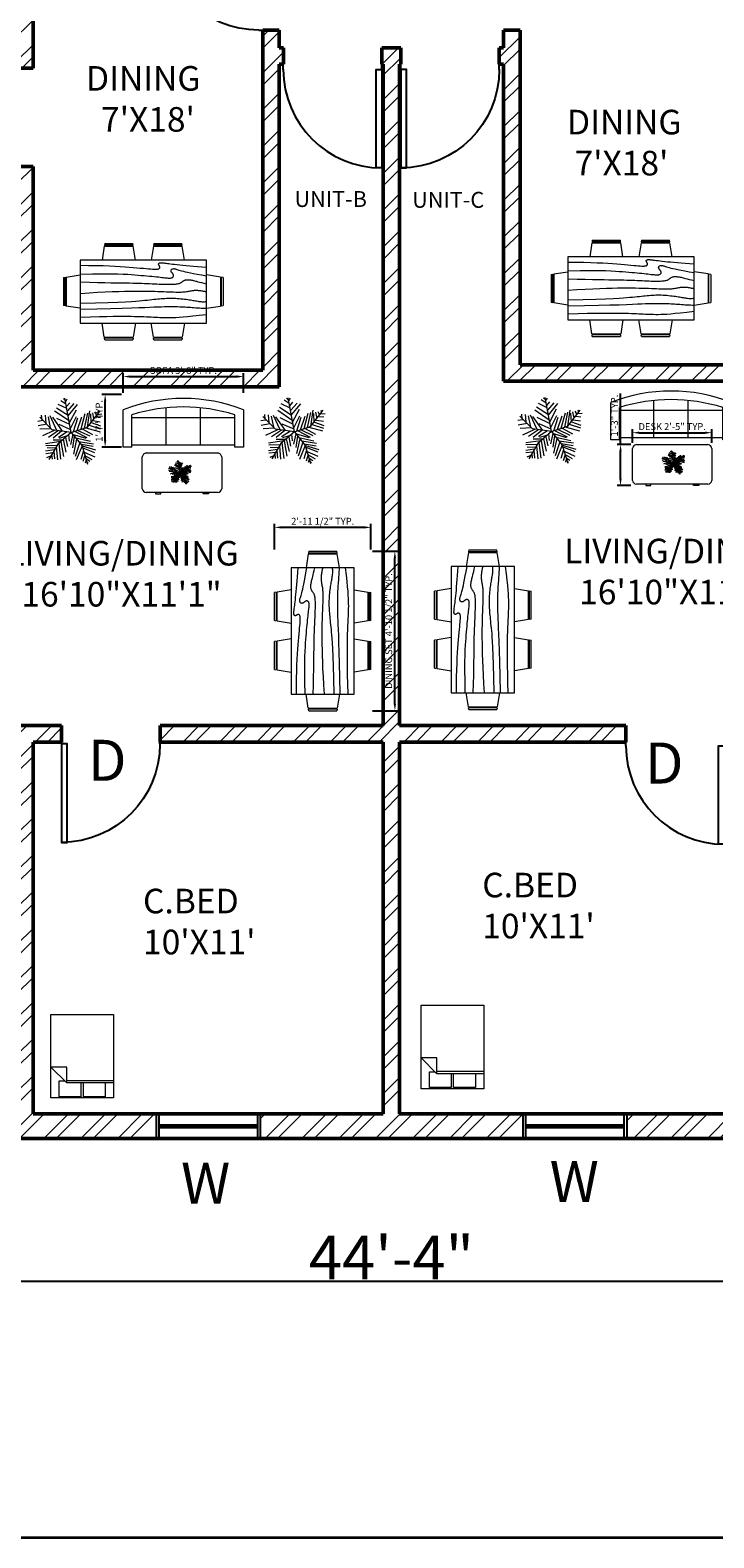
# Model space of a CAD drawing. Units: inches. Extents: x -31842 to -29388, y 18869 to 19743.
# Tile 2 of 12: x -31517 to -31268, y 18869 to 19420. Entities that reach past the tile are written whole.
import ezdxf

# ---------------------------------------------------------------- set-up
doc = ezdxf.new("R2010")
doc.units = ezdxf.units.IN
for name, color, linetype, lineweight in [('A-ANNO-DIMS', 2, 'Continuous', 18), ('A-ANNO-SYMB', 2, 'Continuous', 18), ('A-ANNO-TTLB', 7, 'Continuous', 35), ('A-AREA-IDEN', 3, 'Continuous', 18), ('A-DOOR', 3, 'Continuous', 25), ('A-FURN', 8, 'Continuous', 18), ('A-GLAZ', 4, 'Continuous', 25), ('A-WALL', 7, 'Continuous', 50), ('A-WALL-PATT', 8, 'Continuous', 13), ('L-PLNT', 3, 'Continuous', 13)]:
    doc.layers.add(name, color=color, linetype=linetype, lineweight=lineweight)
doc.styles.get("Standard").update_dxf_attribs({"font": 'arial.ttf'})
doc.dimstyles.new('ISO-25', dxfattribs={"dimtxt": 2.5, "dimasz": 2.5, "dimexe": 1.25, "dimexo": 0.625, "dimtad": 1, "dimdec": 0, "dimlunit": 3, "dimtxsty": 'Standard', "dimcen": 2.5, "dimadec": 0, "dimazin": 0, "dimtfac": 1, "dimtdec": 0, "dimtmove": 0, "dimatfit": 3, "dimfxl": 1, "dimarcsym": 0})

# ---------------------------------------------------------------- blocks, each defined once
blk = doc.blocks.new('*U8')
for p, q in [((0, 0), (0, -100)), ((750, 0), (750, -100))]:
    blk.add_line(p, q)
blk.add_lwpolyline([(0, 0), (0, 750), (43.75, 750), (43.75, 0)], close=True)
blk.add_arc((0, 0), 750, 0, 90)
blk = doc.blocks.new('Bed - Queen')
for p, q in [((0, -80.00003), (0, 0)), ((0, 0), (59.99999, 0)), ((59.99999, 0), (59.99999, -80.00003)), ((0, -14.4), (44.8, -14.4)), ((7.99999, -1.2), (28.79998, -1.2)), ((7.99999, -14.4), (7.99999, -1.2)), ((28.79998, -1.2), (28.79998, -14.4)), ((31.19999, -1.2), (51.99999, -1.2)), ((31.19999, -14.4), (31.19999, -1.2)), ((59.99999, -29.6), (44.8, -14.4)), ((44.8, -14.4), (44.8, -29.6)), ((51.99999, -1.2), (51.99999, -16.4)), ((44.8, -16.8), (0, -16.8)), ((51.99999, -16.4), (46.79936, -16.4)), ((44.8, -29.6), (59.99999, -29.6)), ((59.99999, -80.00003), (0, -80.00003))]:
    blk.add_line(p, q)
blk = doc.blocks.new('Dining Set - 36 x 72 in.')
for p, q in [((-22.2343, 26.00059), (-23.4847, 17.99762)), ((-22.2304, 26), (-5.7608, 26)), ((-22, 27.5), (-22.1562, 26.50042)), ((-5.8416, 26.5), (-22.1534, 26.5)), ((-22, 27.5), (-6, 27.5)), ((-5.8437, 26.49966), (-6, 27.5)), ((-4.5152, 17.99762), (-5.7655, 25.99926)), ((5.7657, 26.00059), (4.5153, 17.99762)), ((5.7696, 26), (22.2392, 26)), ((6, 27.5), (5.8438, 26.50042)), ((22.1584, 26.5), (5.8466, 26.5)), ((6, 27.5), (22, 27.5)), ((22.1563, 26.49966), (22, 27.5)), ((23.4848, 17.99762), (22.2345, 25.99926)), ((36, 18), (-36, 18)), ((-36, 18), (-36, -18)), ((36, -18), (36, 18)), ((-44.0006, 8.23428), (-35.9976, 9.48474)), ((44.0006, 8.23428), (35.9976, 9.48474)), ((-45.5, 8), (-44.5004, 8.15617)), ((-45.5, 8), (-45.5, -8)), ((-44.5, -8.15843), (-44.5, 8.15338)), ((-44, 8.23041), (-44, -8.23915)), ((44, 8.23041), (44, -8.23915)), ((44.5, -8.15843), (44.5, 8.15338)), ((45.5, 8), (44.5005, 8.15617)), ((45.5, 8), (45.5, -8)), ((-44.4997, -8.15631), (-45.5, -8)), ((-35.9976, -9.48476), (-43.9993, -8.2345)), ((35.9976, -9.48476), (43.9993, -8.2345)), ((44.4997, -8.15631), (45.5, -8)), ((-36, -18), (36, -18)), ((-22.2343, -26.0006), (-23.4847, -17.99762)), ((-4.5152, -17.99762), (-5.7655, -25.99928)), ((5.7657, -26.0006), (4.5153, -17.99762)), ((23.4848, -17.99762), (22.2345, -25.99928)), ((-22.2304, -26), (-5.7608, -26)), ((-22, -27.5), (-22.1562, -26.50044)), ((-5.8416, -26.5), (-22.1534, -26.5)), ((-22, -27.5), (-6, -27.5)), ((-5.8437, -26.49967), (-6, -27.5)), ((5.7696, -26), (22.2392, -26)), ((6, -27.5), (5.8438, -26.50044)), ((22.1584, -26.5), (5.8466, -26.5)), ((6, -27.5), (22, -27.5)), ((22.1563, -26.49967), (22, -27.5))]:
    blk.add_line(p, q)
for points in [[(-36, 15), (-31.1772, 14.97754), (-26.8079, 14.91406), (-22.8538, 14.81543), (-19.276, 14.6875), (-16.0362, 14.53613), (-13.0957, 14.36718), (-10.4159, 14.18652), (-7.9583, 14), (-5.6904, 13.81315), (-3.6035, 13.63021), (-1.6954, 13.45508), (0.0365, 13.29166), (1.5945, 13.14388), (2.9811, 13.01562), (4.1988, 12.9108), (5.25, 12.83333), (6.1393, 12.78613), (6.8802, 12.76823), (7.4883, 12.77767), (7.9792, 12.8125), (8.3685, 12.87077), (8.6719, 12.95052), (8.9049, 13.0498), (9.0833, 13.16666), (9.2205, 13.29899), (9.3216, 13.44401), (9.3895, 13.59879), (9.4271, 13.76041), (9.4373, 13.92594), (9.4232, 14.09245), (9.3875, 14.257), (9.3333, 14.41666), (9.2638, 14.56917), (9.1836, 14.71484), (9.0975, 14.85465), (9.0104, 14.98958), (8.9272, 15.1206), (8.8529, 15.2487), (8.7922, 15.37483), (8.75, 15.5), (8.7305, 15.62467), (8.7344, 15.74739), (8.7617, 15.86621), (8.8125, 15.97916), (8.8867, 16.08431), (8.9844, 16.17968), (9.1055, 16.26334), (9.25, 16.33333), (9.4189, 16.38802), (9.6172, 16.42708), (9.8506, 16.45052), (10.125, 16.45833), (10.4463, 16.45052), (10.8203, 16.42708), (11.2529, 16.38802), (11.75, 16.33333), (12.3184, 16.26318), (12.9694, 16.17838), (13.7151, 16.07991), (14.5677, 15.96875), (15.5395, 15.84586), (16.6426, 15.71224), (17.8893, 15.56884), (19.2917, 15.41666), (20.859, 15.25667), (22.5879, 15.08984), (24.4721, 14.91715), (26.5052, 14.73958), (28.6809, 14.5581), (30.9929, 14.3737), (33.4347, 14.18733), (36, 14)], [(-36, 10), (-28.9766, 10.14274), (-23.1725, 10.20442), (-18.4241, 10.19775), (-14.5677, 10.13541), (-11.4399, 10.03011), (-8.877, 9.89453), (-6.7154, 9.74137), (-4.7917, 9.58333), (-2.9698, 9.43082), (-1.2246, 9.28515), (0.4415, 9.14534), (2.026, 9.01041), (3.5266, 8.87939), (4.9408, 8.7513), (6.266, 8.62516), (7.5, 8.5), (8.6411, 8.37549), (9.6914, 8.2539), (10.6538, 8.13818), (11.5312, 8.03125), (12.3267, 7.93603), (13.043, 7.85547), (13.6831, 7.79248), (14.25, 7.75), (14.7471, 7.7303), (15.1797, 7.73307), (15.5537, 7.75732), (15.875, 7.80208), (16.1494, 7.86637), (16.3828, 7.94922), (16.5811, 8.04964), (16.75, 8.16666), (16.8944, 8.29915), (17.0143, 8.44531), (17.1089, 8.60319), (17.1771, 8.77083), (17.218, 8.94629), (17.2305, 9.1276), (17.2137, 9.31282), (17.1667, 9.5), (17.0895, 9.6875), (16.987, 9.875), (16.8649, 10.0625), (16.7292, 10.25), (16.5856, 10.4375), (16.4401, 10.625), (16.2985, 10.8125), (16.1667, 11), (16.05, 11.18733), (15.9518, 11.3737), (15.8752, 11.5581), (15.8229, 11.73958), (15.798, 11.91715), (15.8034, 12.08984), (15.842, 12.25667), (15.9167, 12.41666), (16.0295, 12.56836), (16.1784, 12.70833), (16.3605, 12.83268), (16.5729, 12.9375), (16.8127, 13.01888), (17.0768, 13.07291), (17.3625, 13.0957), (17.6667, 13.08333), (17.9894, 13.03312), (18.3418, 12.94726), (18.7382, 12.82918), (19.1927, 12.68229), (19.7195, 12.51001), (20.3327, 12.31575), (21.0465, 12.10294), (21.875, 11.875), (22.8357, 11.63354), (23.959, 11.37304), (25.2786, 11.08618), (26.8282, 10.76562), (28.6414, 10.40405), (30.752, 9.99414), (33.1936, 9.52856), (36, 9)], [(-36, 5.5), (-30.7157, 5.3348), (-26.069, 5.20963), (-21.9946, 5.11767), (-18.4271, 5.05208), (-15.3009, 5.00602), (-12.5508, 4.97265), (-10.1112, 4.94515), (-7.9167, 4.91666), (-5.909, 4.88167), (-4.0586, 4.83984), (-2.3429, 4.79215), (-0.7396, 4.73958), (0.7739, 4.6831), (2.22, 4.6237), (3.6213, 4.56233), (5, 4.5), (6.373, 4.43782), (7.7344, 4.3776), (9.0723, 4.32129), (10.375, 4.27083), (11.6309, 4.22819), (12.8281, 4.19531), (13.9551, 4.17415), (15, 4.16666), (15.954, 4.17448), (16.819, 4.19791), (17.6001, 4.23698), (18.3021, 4.29166), (18.9299, 4.36198), (19.4883, 4.44791), (19.9823, 4.54948), (20.4167, 4.66666), (20.7969, 4.79899), (21.1302, 4.94401), (21.4245, 5.09879), (21.6875, 5.26041), (21.9271, 5.42594), (22.1511, 5.59245), (22.3672, 5.757), (22.5834, 5.91666), (22.8065, 6.06868), (23.0404, 6.21093), (23.2879, 6.34147), (23.5521, 6.45833), (23.8358, 6.55957), (24.142, 6.64323), (24.4735, 6.70735), (24.8334, 6.75), (25.2235, 6.76969), (25.642, 6.76692), (26.0858, 6.74267), (26.5521, 6.69791), (27.0379, 6.63362), (27.5404, 6.55078), (28.0565, 6.45036), (28.5834, 6.33333), (29.1242, 6.19987), (29.7071, 6.04687), (30.3661, 5.87044), (31.1354, 5.66666), (32.0493, 5.43164), (33.142, 5.16146), (34.4475, 4.85221), (36, 4.5)], [(-36, -1), (-30.7915, -0.6591), (-26.0195, -0.38216), (-21.6519, -0.16284), (-17.6563, 0.00521), (-14.0005, 0.12833), (-10.6523, 0.21289), (-7.5796, 0.26522), (-4.75, 0.29166), (-2.134, 0.29793), (0.2878, 0.28711), (2.5317, 0.26163), (4.6146, 0.22396), (6.5529, 0.17651), (8.3633, 0.12174), (10.0623, 0.06209), (11.6667, 0), (13.1899, -0.06201), (14.6341, -0.1211), (15.9982, -0.17432), (17.2813, -0.21875), (18.4823, -0.25147), (19.6003, -0.26953), (20.6343, -0.27002), (21.5834, -0.25), (22.4481, -0.20768), (23.2357, -0.14584), (23.9549, -0.06836), (24.6146, 0.02083), (25.2235, 0.11784), (25.7904, 0.21875), (26.3241, 0.31966), (26.8334, 0.41666), (27.3265, 0.50618), (27.8099, 0.58593), (28.2894, 0.65397), (28.7709, 0.70833), (29.2601, 0.74707), (29.763, 0.76823), (30.2855, 0.76985), (30.8334, 0.75), (31.4088, 0.70784), (31.9994, 0.64713), (32.589, 0.57275), (33.1615, 0.48958), (33.7008, 0.4025), (34.1908, 0.3164), (34.6153, 0.23616), (34.9584, 0.16666), (35.2099, 0.11165), (35.3848, 0.07031), (35.504, 0.04069), (35.5886, 0.02083), (35.6594, 0.00879), (35.7377, 0.0026), (35.8442, 0.00032), (36, 0)], [(-36, -6.5), (-27.1843, -6.31267), (-20.084, -6.1263), (-14.469, -5.9419), (-10.1094, -5.76042), (-6.7752, -5.58285), (-4.2363, -5.41016), (-2.2629, -5.24333), (-0.625, -5.08334), (0.8708, -4.93099), (2.2715, -4.78646), (3.5872, -4.64974), (4.8281, -4.52084), (6.0046, -4.39974), (7.127, -4.28646), (8.2053, -4.18099), (9.25, -4.08334), (10.2705, -3.99382), (11.2734, -3.91407), (12.2647, -3.84603), (13.25, -3.79167), (14.2354, -3.75293), (15.2266, -3.73177), (16.2295, -3.73015), (17.25, -3.75), (18.2912, -3.79248), (19.3451, -3.85547), (20.4009, -3.93604), (21.4479, -4.03125), (22.4754, -4.13819), (23.4727, -4.25391), (24.4289, -4.37549), (25.3334, -4.5), (26.1785, -4.62492), (26.9694, -4.74935), (27.7145, -4.87281), (28.4219, -4.99479), (29.1, -5.11483), (29.7572, -5.23242), (30.4016, -5.34709), (31.0417, -5.45834), (31.6837, -5.56437), (32.3262, -5.65821), (32.9658, -5.73153), (33.599, -5.77604), (34.2224, -5.78345), (34.8327, -5.74545), (35.4264, -5.65373), (36, -5.5)], [(-36, -10), (-26.4022, -9.81299), (-18.4675, -9.62891), (-11.9839, -9.45069), (-6.7396, -9.28125), (-2.5226, -9.12354), (0.8789, -8.98047), (3.6769, -8.85498), (6.0833, -8.75), (8.2767, -8.66765), (10.3021, -8.60677), (12.1712, -8.56543), (13.8958, -8.54167), (15.4876, -8.53353), (16.9583, -8.53907), (18.3197, -8.55632), (19.5834, -8.58334), (20.7616, -8.61841), (21.8685, -8.66081), (22.9188, -8.71004), (23.9271, -8.76563), (24.9081, -8.82707), (25.8763, -8.89388), (26.8465, -8.96558), (27.8334, -9.04167), (28.8474, -9.12118), (29.8828, -9.20117), (30.93, -9.27824), (31.9792, -9.34896), (33.0205, -9.40991), (34.0443, -9.45768), (35.0407, -9.48885), (36, -9.5)], [(-36, -14.5), (-30.0881, -14.33513), (-25.0332, -14.21224), (-20.7312, -14.12647), (-17.0781, -14.07292), (-13.97, -14.04671), (-11.3027, -14.04297), (-8.9724, -14.05681), (-6.875, -14.08334), (-4.9224, -14.11833), (-3.0905, -14.16016), (-1.3709, -14.20785), (0.2448, -14.26042), (1.7647, -14.3169), (3.1973, -14.3763), (4.5507, -14.43767), (5.8333, -14.5), (7.0554, -14.5621), (8.235, -14.62175), (9.3922, -14.67652), (10.5469, -14.72396), (11.7192, -14.76164), (12.929, -14.78711), (14.1965, -14.79794), (15.5417, -14.79167), (16.9933, -14.76424), (18.6152, -14.70508), (20.4804, -14.60197), (22.6615, -14.44271), (25.2312, -14.21509), (28.2624, -13.9069), (31.8277, -13.50594), (36, -13)]]:
    blk.add_lwpolyline(points)
blk = doc.blocks.new('Desk - 30 x 60 in.')
for p, q in [((-26.999995, 0), (26.999995, 0)), ((-29.999995, -27), (-29.999995, -3)), ((29.999995, -3), (29.999995, -27)), ((26.999995, -30), (-26.999995, -30)), ((-20.000005, -30), (-20.000005, -31)), ((-20.000005, -31), (-16.000005, -31)), ((-16.000005, -31), (-16.000005, -30)), ((15.999995, -31), (15.999995, -30)), ((19.999995, -31), (15.999995, -31)), ((19.999995, -30), (19.999995, -31))]:
    blk.add_line(p, q)
for centre, start, end in [((-26.499995, -3.5), 98.1301, 171.8699), ((26.499995, -3.5), 8.130102, 81.8699), ((-26.499995, -26.5), 188.1301, 261.8699), ((26.499995, -26.5), 278.1301, 351.8699)]:
    blk.add_arc(centre, 3.535534, start, end)
blk = doc.blocks.new('Sofa - Roundback 7 ft.')
for p, q in [((-12.00002, -32.4421), (-12.00003, -6.5971)), ((11.99997, -32.4421), (11.99998, -6.5971)), ((-36.000027, -34), (-36.000027, -11.4696)), ((-35.999844, -13.3819), (35.9998, -13.3819)), ((35.99998, -34), (35.99998, -11.4696)), ((-36.000027, -32.4421), (35.99998, -32.4421))]:
    blk.add_line(p, q)
for points in [[(-36.000027, -34), (-42.000027, -34), (-42.000027, -8)], [(41.99998, -8), (41.99998, -34), (35.99998, -34)]]:
    blk.add_lwpolyline(points)
for centre, radius, start, end in [((0, -114.25), 114.25, 68.43141, 111.5686), ((-0.00001, -127.1968), 121.1968, 72.72033, 107.2797)]:
    blk.add_arc(centre, radius, start, end)
blk = doc.blocks.new('*U122')
for p, q in [((-221.9198, 1197.3052), (-433.5526, 1338.8594)), ((-258.7244, 1362.456), (-332.3336, 1421.4348)), ((0, 0), (-266.7, 1447.8)), ((-231.1146, 1315.2628), (-166.7002, 1421.4348)), ((-800.1, 114.3), (-1333.5, 647.7)), ((-1234.059, 536.7274), (-1252.4486, 737.2604)), ((-1105.2302, 725.4494), (-1077.6458, 395.1732)), ((-976.4268, 666.4706), (-884.4026, 194.6402)), ((-902.8176, 713.6638), (-617.5756, 100.2538)), ((-369.1382, 53.086), (-783.1836, 642.874)), ((-93.091, 489.5342), (-700.3796, 902.3858)), ((-129.8956, 713.6638), (-626.7704, 1032.1544)), ((-185.1152, 1008.5578), (-553.1612, 1185.4942)), ((-194.31, 1102.9442), (-65.4812, 1256.284)), ((-148.3106, 914.1968), (118.5418, 1220.9018)), ((-129.8956, 701.8528), (265.7602, 1185.4942)), ((-74.7014, 418.7444), (219.7608, 961.39)), ((-28.6766, 171.0436), (228.9556, 678.2816)), ((256.5654, 88.4682), (449.7832, 666.4706)), ((412.9786, 147.447), (587.8068, 796.2392)), ((560.197, 182.8292), (698.2206, 819.8358)), ((685.8, 228.6), (1219.2, 914.4)), ((689.0258, 230.0224), (790.2448, 914.1968)), ((808.6344, 784.4282), (827.0494, 418.7444)), ((891.4384, 831.6214), (946.658, 572.1096)), ((983.4626, 867.0036), (1066.2666, 725.4494)), ((1029.462, 654.685), (1241.0948, 631.0884)), ((1112.2914, 760.8316), (1296.3144, 784.4282)), ((1121.4862, 925.9824), (1149.0706, 831.6214)), ((-1206.4492, 501.3198), (-1418.082, 465.9376)), ((-1031.621, 347.98), (-1399.667, 277.1902)), ((-847.598, 159.2326), (-1326.0578, 135.636)), ((-718.7946, 88.4682), (-1215.644, -147.447)), ((-543.9664, 76.6572), (-967.2066, -206.4512)), ((0, 0), (-800.1, 114.3)), ((-405.9428, 53.086), (-764.794, -241.8334)), ((-617.5756, 607.4918), (-74.7014, 347.98)), ((0, 0), (-571.5, -495.3)), ((-166.7002, 29.4894), (-543.9664, -206.4512)), ((-525.5514, 347.98), (-28.6766, 123.8504)), ((0, 0), (685.8, 228.6)), ((0, 0), (457.2, -571.5)), ((100.1268, 41.275), (284.1498, 619.2774)), ((164.5412, 41.275), (661.416, -218.2368)), ((284.1498, 88.4682), (781.0246, -147.447)), ((458.978, 147.447), (891.4384, -88.4682)), ((615.4166, 194.6402), (1185.8752, 41.275)), ((753.4148, 312.5978), (1222.6798, 159.2326)), ((845.439, 418.7444), (1241.0948, 277.1902)), ((919.0482, 501.3198), (1222.6798, 454.152)), ((-442.7474, -383.3876), (-1086.8406, -477.7486)), ((-617.5756, -548.5384), (-1077.6458, -560.324)), ((-571.5, -495.3), (-952.5, -1143)), ((-387.5278, -324.4088), (-764.794, -324.4088)), ((-635.9652, -607.5172), (-580.771, -1150.1374)), ((-525.5514, -465.963), (-451.9422, -1126.5408)), ((-166.7002, -147.447), (-507.1618, -253.619)), ((-433.5526, -383.3876), (-323.1134, -1020.3688)), ((-341.5284, -289.0012), (-221.9198, -831.6214)), ((-240.3094, -218.2368), (-157.5054, -595.7062)), ((-120.7008, -88.4682), (-93.091, -371.5766)), ((63.3222, -76.6826), (-37.8714, -513.1308)), ((44.9326, -64.897), (615.4166, -241.8334)), ((127.7366, -159.258), (54.1274, -654.685)), ((228.9556, -289.0012), (90.932, -914.1968)), ((357.759, -430.5554), (164.5412, -1020.3688)), ((192.151, -230.0224), (817.8292, -371.5766)), ((458.978, -572.1096), (210.5406, -1161.923)), ((311.7596, -383.3876), (937.4378, -477.7486)), ((412.9786, -501.3452), (919.0482, -583.9206)), ((457.2, -571.5), (685.8, -1333.5)), ((468.1982, -572.1096), (1029.462, -737.2604)), ((-718.7946, -737.2604), (-1086.8406, -796.2392)), ((-783.1836, -867.029), (-1077.6458, -902.4112)), ((-875.2078, -1008.5832), (-1040.8412, -1079.3476)), ((-681.9646, -666.496), (-1022.4262, -654.685)), ((-829.2084, -937.7934), (-810.7934, -1126.5408)), ((-737.1842, -784.4536), (-709.5744, -1114.7298)), ((514.1976, -772.6426), (403.7838, -1138.3264)), ((486.5878, -642.8994), (983.4626, -843.4324)), ((578.612, -961.39), (495.7826, -1232.7128)), ((541.8074, -831.6214), (992.6574, -1032.1544)), ((578.612, -973.1756), (873.0488, -1138.3264)), ((624.6114, -1161.923), (587.8068, -1291.6916)), ((624.6114, -1102.9442), (781.0246, -1209.1162)), ((679.8056, -1268.095), (716.6102, -1291.6916))]:
    blk.add_line(p, q)
blk = doc.blocks.new('*D197')
at = {"layer": 'A-ANNO-DIMS', "color": 0, "lineweight": -2, "transparency": 16777216}
for p, q in [((-31651.45, 19014.34), (-31651.45, 18961.52)), ((-31119.45, 19014.34), (-31119.45, 18961.52)), ((-31648.95, 18962.77), (-31121.95, 18962.77))]:
    blk.add_line(p, q, dxfattribs=at)
at = {"layer": 'A-ANNO-DIMS', "color": 0, "transparency": 16777216}
for points in [[(-31648.95, 18963.19), (-31648.95, 18962.35), (-31651.45, 18962.77)], [(-31121.95, 18963.19), (-31121.95, 18962.35), (-31119.45, 18962.77)]]:
    blk.add_solid(points, dxfattribs=at)
at = {"layer": 'Defpoints', "color": 0, "transparency": 16777216}
for p in [(-31651.45, 19014.96), (-31119.45, 19014.96), (-31119.45, 18962.77)]:
    blk.add_point(p, dxfattribs=at)
at = {"layer": 'A-ANNO-DIMS', "color": 0, "transparency": 16777216, "insert": (-31385.45, 18971.4), "char_height": 2.5, "attachment_point": 5}
blk.add_mtext('{\\H6.4x;44\'-4"}', dxfattribs=at)
blk = doc.blocks.new('WIN-3FT')
for p, q in [((0, 36), (9, 36)), ((4, 0), (4, 36)), ((4.5, 0), (4.5, 36)), ((5, 0), (5, 36)), ((0, 0), (9, 0))]:
    blk.add_line(p, q)
blk = doc.blocks.new('*D241')
at = {"layer": 'A-ANNO-DIMS', "color": 0, "lineweight": -2, "transparency": 16777216}
for p, q in [((-31392.32, 19229.74), (-31382.94, 19229.74)), ((-31384.19, 19173.9), (-31384.19, 19227.24)), ((-31392.32, 19171.4), (-31382.94, 19171.4))]:
    blk.add_line(p, q, dxfattribs=at)
at = {"layer": 'A-ANNO-DIMS', "color": 0, "transparency": 16777216}
for points in [[(-31384.61, 19227.24), (-31383.77, 19227.24), (-31384.19, 19229.74)], [(-31384.61, 19173.9), (-31383.77, 19173.9), (-31384.19, 19171.4)]]:
    blk.add_solid(points, dxfattribs=at)
at = {"layer": 'Defpoints', "color": 0, "transparency": 16777216}
for p in [(-31392.94, 19229.74), (-31384.19, 19229.74), (-31392.94, 19171.4)]:
    blk.add_point(p, dxfattribs=at)
at = {"layer": 'A-ANNO-DIMS', "color": 0, "transparency": 16777216, "insert": (-31386.11, 19200.57), "char_height": 2.5, "attachment_point": 5, "rotation": 90}
blk.add_mtext('DINING SET 4\'-10 1/2" TYP.', dxfattribs=at)
blk = doc.blocks.new('*D242')
at = {"layer": 'A-ANNO-DIMS', "color": 0, "lineweight": -2, "transparency": 16777216}
for p, q in [((-31428.21, 19230.36), (-31428.21, 19239.74)), ((-31392.94, 19230.36), (-31392.94, 19239.74)), ((-31395.44, 19238.49), (-31425.71, 19238.49))]:
    blk.add_line(p, q, dxfattribs=at)
at = {"layer": 'A-ANNO-DIMS', "color": 0, "transparency": 16777216}
for points in [[(-31425.71, 19238.91), (-31425.71, 19238.07), (-31428.21, 19238.49)], [(-31395.44, 19238.91), (-31395.44, 19238.07), (-31392.94, 19238.49)]]:
    blk.add_solid(points, dxfattribs=at)
at = {"layer": 'Defpoints', "color": 0, "transparency": 16777216}
for p in [(-31428.21, 19238.49), (-31428.21, 19229.74), (-31392.94, 19229.74)]:
    blk.add_point(p, dxfattribs=at)
at = {"layer": 'A-ANNO-DIMS', "color": 0, "transparency": 16777216, "insert": (-31410.57, 19240.41), "char_height": 2.5, "attachment_point": 5}
blk.add_mtext('2\'-11 1/2" TYP.', dxfattribs=at)
blk = doc.blocks.new('*D247')
at = {"layer": 'A-ANNO-DIMS', "color": 0, "lineweight": -2, "transparency": 16777216}
for p, q in [((-31297.36, 19269.39), (-31297.36, 19274.38)), ((-31294.86, 19273.13), (-31270.81, 19273.13)), ((-31268.31, 19269.39), (-31268.31, 19274.38))]:
    blk.add_line(p, q, dxfattribs=at)
at = {"layer": 'A-ANNO-DIMS', "color": 0, "transparency": 16777216}
for points in [[(-31294.86, 19273.54), (-31294.86, 19272.71), (-31297.36, 19273.13)], [(-31270.81, 19273.54), (-31270.81, 19272.71), (-31268.31, 19273.13)]]:
    blk.add_solid(points, dxfattribs=at)
at = {"layer": 'Defpoints', "color": 0, "transparency": 16777216}
for p in [(-31268.31, 19273.13), (-31297.36, 19268.77), (-31268.31, 19268.77)]:
    blk.add_point(p, dxfattribs=at)
at = {"layer": 'A-ANNO-DIMS', "color": 0, "transparency": 16777216, "insert": (-31282.84, 19275.04), "char_height": 2.5, "attachment_point": 5}
blk.add_mtext('DESK 2\'-5" TYP.', dxfattribs=at)
blk = doc.blocks.new('*D248')
at = {"layer": 'A-ANNO-DIMS', "color": 0, "lineweight": -2, "transparency": 16777216}
for p, q in [((-31301.72, 19268.77), (-31301.72, 19287.52)), ((-31297.99, 19268.77), (-31302.97, 19268.77)), ((-31301.72, 19256.26), (-31301.72, 19266.27)), ((-31297.99, 19253.76), (-31302.97, 19253.76))]:
    blk.add_line(p, q, dxfattribs=at)
at = {"layer": 'A-ANNO-DIMS', "color": 0, "transparency": 16777216}
for points in [[(-31302.14, 19266.27), (-31301.3, 19266.27), (-31301.72, 19268.77)], [(-31302.14, 19256.26), (-31301.3, 19256.26), (-31301.72, 19253.76)]]:
    blk.add_solid(points, dxfattribs=at)
at = {"layer": 'Defpoints', "color": 0, "transparency": 16777216}
for p in [(-31301.72, 19268.77), (-31297.36, 19268.77), (-31297.36, 19253.76)]:
    blk.add_point(p, dxfattribs=at)
at = {"layer": 'A-ANNO-DIMS', "color": 0, "transparency": 16777216, "insert": (-31303.62, 19279.39), "char_height": 2.5, "attachment_point": 5, "rotation": 90}
blk.add_mtext('1\'-3" TYP.', dxfattribs=at)
blk = doc.blocks.new('*D253')
at = {"layer": 'A-ANNO-DIMS', "color": 0, "lineweight": -2, "transparency": 16777216}
for p, q in [((-31483.49, 19287.69), (-31483.49, 19294.91)), ((-31439.5, 19287.69), (-31439.5, 19294.91)), ((-31480.99, 19293.66), (-31442, 19293.66))]:
    blk.add_line(p, q, dxfattribs=at)
at = {"layer": 'A-ANNO-DIMS', "color": 0, "transparency": 16777216}
for points in [[(-31480.99, 19294.08), (-31480.99, 19293.25), (-31483.49, 19293.66)], [(-31442, 19294.08), (-31442, 19293.25), (-31439.5, 19293.66)]]:
    blk.add_solid(points, dxfattribs=at)
at = {"layer": 'Defpoints', "color": 0, "transparency": 16777216}
for p in [(-31439.5, 19293.66), (-31483.49, 19287.06), (-31439.5, 19287.06)]:
    blk.add_point(p, dxfattribs=at)
at = {"layer": 'A-ANNO-DIMS', "color": 0, "transparency": 16777216, "insert": (-31461.5, 19295.58), "char_height": 2.5, "attachment_point": 5}
blk.add_mtext('SOFA 3\'-8" TYP.', dxfattribs=at)
blk = doc.blocks.new('*D254')
at = {"layer": 'A-ANNO-DIMS', "color": 0, "lineweight": -2, "transparency": 16777216}
for p, q in [((-31484.12, 19287.06), (-31491.34, 19287.06)), ((-31490.09, 19270.36), (-31490.09, 19284.56)), ((-31484.12, 19267.86), (-31491.34, 19267.86))]:
    blk.add_line(p, q, dxfattribs=at)
at = {"layer": 'A-ANNO-DIMS', "color": 0, "transparency": 16777216}
for points in [[(-31490.51, 19284.56), (-31489.68, 19284.56), (-31490.09, 19287.06)], [(-31490.51, 19270.36), (-31489.68, 19270.36), (-31490.09, 19267.86)]]:
    blk.add_solid(points, dxfattribs=at)
at = {"layer": 'Defpoints', "color": 0, "transparency": 16777216}
for p in [(-31490.09, 19287.06), (-31483.49, 19287.06), (-31483.49, 19267.86)]:
    blk.add_point(p, dxfattribs=at)
at = {"layer": 'A-ANNO-DIMS', "color": 0, "transparency": 16777216, "insert": (-31491.98, 19277.46), "char_height": 2.5, "attachment_point": 5, "rotation": 90}
blk.add_mtext('1\'-7" TYP.', dxfattribs=at)

msp = doc.modelspace()

# ---------------------------------------------------------------- hatches: boundary and pattern name
at = {"layer": 'A-WALL-PATT'}
h = msp.add_hatch(dxfattribs=at)
h.set_pattern_fill('ANSI32', color=256)
h.paths.add_polyline_path([(-31119.45, 19656.96), (-31254.45, 19656.96), (-31254.45, 19614.96), (-31277.45, 19614.96), (-31277.45, 19605.96), (-31254.45, 19605.96), (-31254.45, 19555.2), (-31248.45, 19555.2), (-31248.45, 19605.96), (-31240.75, 19605.96), (-31240.75, 19614.96), (-31248.45, 19614.96), (-31248.45, 19650.96), (-31128.45, 19650.96), (-31128.45, 19614.96), (-31216.75, 19614.96), (-31216.75, 19605.96), (-31128.45, 19605.96), (-31128.45, 19559.96), (-31119.45, 19559.96)])
h.paths.add_polyline_path([(-31153.94, 19473.06), (-31153.92, 19475.96), (-31248.45, 19475.96), (-31248.45, 19519.2), (-31251.45, 19519.2), (-31254.45, 19519.2), (-31254.45, 19497.96), (-31267.62, 19497.96), (-31267.62, 19491.96), (-31254.45, 19491.96), (-31254.45, 19465.12), (-31248.45, 19465.12), (-31248.45, 19469.96), (-31161.45, 19469.96), (-31161.45, 19458.96), (-31155.45, 19458.96), (-31155.45, 19469.96), (-31153.94, 19469.96)])
h.paths.add_polyline_path([(-31119.45, 19521.96), (-31128.45, 19521.96), (-31128.45, 19475.96), (-31129.92, 19475.96), (-31129.92, 19469.96), (-31128.45, 19469.96), (-31128.45, 19421.96), (-31155.45, 19421.96), (-31155.45, 19432.96), (-31161.45, 19432.96), (-31161.45, 19421.96), (-31248.45, 19421.96), (-31248.45, 19441.12), (-31254.45, 19441.12), (-31254.45, 19406.17), (-31248.45, 19406.17), (-31248.45, 19415.96), (-31128.45, 19415.96), (-31128.45, 19375.96), (-31119.45, 19375.96)])
h.paths.add_polyline_path([(-31315.45, 19614.96), (-31366.45, 19614.96), (-31366.45, 19605.96), (-31344.45, 19605.96), (-31344.45, 19456.39), (-31338.45, 19456.39), (-31338.45, 19491.96), (-31328.43, 19491.96), (-31328.43, 19497.96), (-31338.45, 19497.96), (-31338.45, 19605.96), (-31315.45, 19605.96)])
h.paths.add_polyline_path([(-31404.45, 19614.96), (-31455.1, 19614.96), (-31455.1, 19605.96), (-31432.45, 19605.96), (-31432.45, 19497.96), (-31448.67, 19497.96), (-31448.67, 19491.96), (-31432.45, 19491.96), (-31432.45, 19456.39), (-31429.07, 19456.39), (-31426.45, 19456.39), (-31426.45, 19605.96), (-31404.45, 19605.96)])
h.paths.add_polyline_path([(-31493.1, 19614.96), (-31516.45, 19614.96), (-31516.45, 19656.96), (-31651.45, 19656.96), (-31651.45, 19559.96), (-31642.45, 19559.96), (-31642.45, 19605.96), (-31556.65, 19605.96), (-31556.65, 19614.96), (-31642.45, 19614.96), (-31642.45, 19650.96), (-31522.45, 19650.96), (-31522.45, 19614.96), (-31532.65, 19614.96), (-31532.65, 19613.66), (-31532.65, 19610.46), (-31532.65, 19605.96), (-31522.45, 19605.96), (-31522.45, 19541.95), (-31516.45, 19541.95), (-31516.45, 19605.96), (-31493.1, 19605.96)])
h.paths.add_polyline_path([(-31642.45, 19521.96), (-31651.45, 19521.96), (-31651.45, 19374.96), (-31642.45, 19374.96), (-31642.45, 19415.96), (-31522.45, 19415.96), (-31522.45, 19406.54), (-31516.45, 19406.54), (-31516.45, 19441.56), (-31522.45, 19441.56), (-31522.45, 19421.96), (-31609.45, 19421.96), (-31609.45, 19432.96), (-31615.45, 19432.96), (-31615.45, 19421.96), (-31642.45, 19421.96), (-31642.45, 19469.96), (-31641.6, 19469.96), (-31641.6, 19475.96), (-31642.45, 19475.96)])
h.paths.add_polyline_path([(-31516.45, 19491.96), (-31506.54, 19491.96), (-31506.54, 19497.96), (-31516.45, 19497.96), (-31516.45, 19505.95), (-31522.45, 19505.95), (-31522.45, 19475.96), (-31617.6, 19475.96), (-31617.6, 19469.96), (-31615.45, 19469.96), (-31615.45, 19458.96), (-31609.45, 19458.96), (-31609.45, 19469.96), (-31522.45, 19469.96), (-31522.45, 19465.56), (-31516.45, 19465.56)])
h.paths.add_polyline_path([(-31248.45, 19370.17), (-31251.45, 19370.17), (-31254.45, 19370.17), (-31254.45, 19297.96), (-31338.45, 19297.96), (-31338.45, 19420.39), (-31344.45, 19420.39), (-31344.45, 19413.96), (-31346.02, 19413.96), (-31346.02, 19407.96), (-31344.45, 19407.96), (-31344.45, 19291.96), (-31213.45, 19291.96), (-31213.45, 19275.43), (-31207.45, 19275.43), (-31207.45, 19291.96), (-31128.45, 19291.96), (-31128.45, 19274.96), (-31119.45, 19274.96), (-31119.45, 19337.96), (-31128.45, 19337.96), (-31128.45, 19297.96), (-31248.45, 19297.96)])
h.paths.add_polyline_path([(-31426.45, 19407.96), (-31424.99, 19407.96), (-31424.99, 19410.83), (-31424.95, 19413.96), (-31426.45, 19413.96), (-31426.45, 19420.39), (-31432.45, 19420.39), (-31432.45, 19295.96), (-31516.45, 19295.96), (-31516.45, 19370.54), (-31522.45, 19370.54), (-31522.45, 19295.96), (-31642.45, 19295.96), (-31642.45, 19336.96), (-31651.45, 19336.96), (-31651.45, 19272.96), (-31642.45, 19272.96), (-31642.45, 19289.96), (-31563.45, 19289.96), (-31563.45, 19270.05), (-31557.45, 19270.05), (-31557.45, 19289.96), (-31426.45, 19289.96)])
h.paths.add_polyline_path([(-31557.45, 19222.83), (-31563.45, 19222.83), (-31563.45, 19217.96), (-31642.45, 19217.96), (-31642.45, 19234.96), (-31651.45, 19234.96), (-31651.45, 19201.96), (-31642.45, 19201.96), (-31642.45, 19211.96), (-31563.45, 19211.96), (-31563.45, 19206.27), (-31562.72, 19206.27), (-31559.53, 19206.27), (-31557.45, 19206.18)])
h.paths.add_polyline_path([(-31553.97, 19163.65), (-31553.95, 19165.96), (-31557.45, 19165.96), (-31557.45, 19182.18), (-31563.45, 19182.18), (-31563.45, 19165.96), (-31639.16, 19165.96), (-31639.16, 19159.96), (-31630.45, 19159.96), (-31630.45, 19110.96), (-31624.45, 19110.96), (-31624.45, 19159.96), (-31553.97, 19159.96)])
h.paths.add_polyline_path([(-31663.16, 19165.96), (-31681.45, 19165.96), (-31681.45, 19014.96), (-31592.45, 19014.96), (-31592.45, 19023.96), (-31624.45, 19023.96), (-31624.45, 19072.96), (-31630.45, 19072.96), (-31630.45, 19023.96), (-31675.45, 19023.96), (-31675.45, 19159.96), (-31663.16, 19159.96)])
h.paths.add_polyline_path([(-31516.45, 19159.96), (-31505.99, 19159.96), (-31505.99, 19165.96), (-31524.95, 19165.96), (-31524.95, 19159.96), (-31522.45, 19159.96), (-31522.45, 19023.96), (-31554.45, 19023.96), (-31554.45, 19014.96), (-31471.45, 19014.96), (-31471.45, 19023.96), (-31516.45, 19023.96)])
h.paths.add_polyline_path([(-31337.45, 19023.96), (-31382.45, 19023.96), (-31382.45, 19159.96), (-31299.75, 19159.96), (-31299.75, 19165.96), (-31344.45, 19165.96), (-31382.45, 19165.96), (-31382.45, 19407.96), (-31382.02, 19413.96), (-31388.95, 19413.96), (-31388.95, 19407.96), (-31388.45, 19407.96), (-31388.45, 19165.96), (-31432.45, 19165.96), (-31469.99, 19165.96), (-31469.99, 19159.96), (-31432.45, 19159.96), (-31388.45, 19159.96), (-31388.45, 19023.96), (-31433.45, 19023.96), (-31433.45, 19014.96), (-31337.45, 19014.96)])
h.paths.add_polyline_path([(-31216.45, 19023.96), (-31248.45, 19023.96), (-31248.45, 19159.96), (-31245.93, 19159.96), (-31245.93, 19162.87), (-31245.93, 19165.96), (-31254.45, 19165.96), (-31263.75, 19165.96), (-31263.75, 19159.96), (-31254.45, 19159.96), (-31254.45, 19023.96), (-31299.45, 19023.96), (-31299.45, 19014.96), (-31216.45, 19014.96)])
h.paths.add_polyline_path([(-31089.45, 19165.96), (-31110.75, 19165.96), (-31110.75, 19159.96), (-31095.45, 19159.96), (-31095.45, 19023.96), (-31140.45, 19023.96), (-31140.45, 19072.96), (-31146.45, 19072.96), (-31146.45, 19023.96), (-31178.45, 19023.96), (-31178.45, 19014.96), (-31089.45, 19014.96)])
h.paths.add_polyline_path([(-31134.75, 19165.96), (-31207.45, 19165.96), (-31207.45, 19182.5), (-31213.45, 19182.5), (-31213.45, 19165.96), (-31216.93, 19165.96), (-31216.93, 19159.96), (-31146.45, 19159.96), (-31146.45, 19110.96), (-31140.45, 19110.96), (-31140.45, 19159.96), (-31134.75, 19159.96)])
h.paths.add_polyline_path([(-31119.45, 19236.96), (-31128.45, 19236.96), (-31128.45, 19219.96), (-31207.45, 19219.96), (-31207.45, 19227.12), (-31213.45, 19227.12), (-31213.45, 19206.5), (-31207.45, 19206.5), (-31207.45, 19213.96), (-31128.45, 19213.96), (-31128.45, 19202.96), (-31119.45, 19202.96)])

# ---------------------------------------------------------------- linework, layer by layer
at = {"layer": 'A-ANNO-TTLB'}
msp.add_lwpolyline([(-31842.18, 19743.36), (-29387.67, 19743.36), (-29387.67, 18868.82), (-31842.18, 18868.82)], close=True, dxfattribs=at)
at = {"layer": 'A-GLAZ'}
for p, q in [((-31471.45, 19023.96), (-31471.45, 19014.96)), ((-31433.45, 19023.96), (-31433.45, 19014.96)), ((-31337.45, 19023.96), (-31337.45, 19014.96)), ((-31299.45, 19023.96), (-31299.45, 19014.96))]:
    msp.add_line(p, q, dxfattribs=at)
at = {"layer": 'A-WALL'}
for p, q in [((-31516.45, 19406.54), (-31516.45, 19441.56)), ((-31432.45, 19295.96), (-31432.45, 19420.39)), ((-31426.45, 19420.39), (-31432.45, 19420.39)), ((-31426.45, 19413.96), (-31426.45, 19420.39)), ((-31344.45, 19420.39), (-31338.45, 19420.39)), ((-31344.45, 19420.39), (-31344.45, 19413.96)), ((-31338.45, 19420.39), (-31338.45, 19297.96)), ((-31426.45, 19413.96), (-31424.95, 19413.96)), ((-31424.95, 19407.96), (-31424.95, 19413.96)), ((-31388.95, 19407.96), (-31388.95, 19413.96)), ((-31388.95, 19413.96), (-31382.02, 19413.96)), ((-31382.02, 19407.96), (-31382.02, 19413.96)), ((-31346.02, 19407.96), (-31346.02, 19413.96)), ((-31346.02, 19413.96), (-31344.45, 19413.96)), ((-31522.45, 19406.54), (-31516.45, 19406.54)), ((-31426.45, 19407.96), (-31424.95, 19407.96)), ((-31426.45, 19289.96), (-31426.45, 19407.96)), ((-31388.95, 19407.96), (-31388.45, 19407.96)), ((-31388.45, 19165.96), (-31388.45, 19407.96)), ((-31382.45, 19165.96), (-31382.45, 19407.96)), ((-31382.45, 19407.96), (-31382.02, 19407.96)), ((-31346.02, 19407.96), (-31344.45, 19407.96)), ((-31344.45, 19407.96), (-31344.45, 19291.96)), ((-31522.45, 19370.54), (-31516.45, 19370.54)), ((-31516.45, 19295.96), (-31516.45, 19370.54)), ((-31516.45, 19295.96), (-31432.45, 19295.96)), ((-31338.45, 19297.96), (-31254.45, 19297.96)), ((-31557.45, 19289.96), (-31426.45, 19289.96)), ((-31344.45, 19291.96), (-31213.45, 19291.96)), ((-31524.95, 19165.96), (-31505.99, 19165.96)), ((-31505.99, 19159.96), (-31505.99, 19165.96)), ((-31469.99, 19159.96), (-31469.99, 19165.96)), ((-31469.99, 19165.96), (-31432.45, 19165.96)), ((-31432.45, 19165.96), (-31388.45, 19165.96)), ((-31382.45, 19165.96), (-31344.45, 19165.96)), ((-31344.45, 19165.96), (-31299.75, 19165.96)), ((-31299.75, 19159.96), (-31299.75, 19165.96)), ((-31516.45, 19023.96), (-31516.45, 19159.96)), ((-31516.45, 19159.96), (-31505.99, 19159.96)), ((-31469.99, 19159.96), (-31432.45, 19159.96)), ((-31432.45, 19159.96), (-31388.45, 19159.96)), ((-31388.45, 19023.96), (-31388.45, 19159.96)), ((-31382.45, 19023.96), (-31382.45, 19159.96)), ((-31382.45, 19159.96), (-31299.75, 19159.96)), ((-31388.45, 19023.96), (-31516.45, 19023.96)), ((-31254.45, 19023.96), (-31382.45, 19023.96)), ((-31089.45, 19014.96), (-31681.45, 19014.96))]:
    msp.add_line(p, q, dxfattribs=at)

# ---------------------------------------------------------------- block references
at = {"layer": 'A-DOOR'}
for p, xscale, yscale, zscale, rotation in [((-31433.87, 19456.39), -0.0480027575407148, 0.0480027575407148, 0.0480027575407148, 90), ((-31388.95, 19406.02), 0.0480441834329324, 0.0480441834329324, 0.0480441834329324, 180), ((-31382.02, 19406.01), -0.0480000000000066, 0.0480000000000066, 0.0480000000000066, 180), ((-31506.05, 19159.25), -0.0480000000000066, 0.0480000000000066, 0.0480000000000066, 180), ((-31263.75, 19158.56), 0.0480000000000001, 0.0480000000000001, 0.0480000000000001, 180)]:
    msp.add_blockref('*U8', p, dxfattribs=dict(at, xscale=xscale, yscale=yscale, zscale=zscale, rotation=rotation))
at = {"layer": 'A-FURN'}
for name, p, xscale, yscale, zscale in [('Dining Set - 36 x 72 in.', (-31476.15, 19324.74), 0.6411469310309978, 0.6411469310309978, 0.6411469310309978), ('Dining Set - 36 x 72 in.', (-31297.92, 19325.91), 0.6411469310309978, 0.6411469310309978, 0.6411469310309978), ('Sofa - Roundback 7 ft.', (-31283.23, 19288.36), 0.5237896943857897, 0.5237896943857897, 0.5237896943857897), ('Sofa - Roundback 7 ft.', (-31461.5, 19285.67), 0.5237896943857897, 0.5237896943857897, 0.5237896943857897), ('Desk - 30 x 60 in.', (-31282.84, 19268.77), 0.4841868825535263, 0.4841868825535263, 0.4841868825535263), ('Desk - 30 x 60 in.', (-31462.01, 19265.72), 0.4841868825535263, 0.4841868825535263, 0.4841868825535263)]:
    msp.add_blockref(name, p, dxfattribs=dict(at, xscale=xscale, yscale=yscale, zscale=zscale))
for name, p, xscale, yscale, zscale, rotation in [('Dining Set - 36 x 72 in.', (-31410.57, 19200.57), 0.6411469310309978, 0.6411469310309978, 0.6411469310309978, 90), ('Dining Set - 36 x 72 in.', (-31352.05, 19201.06), 0.6411469310309978, 0.6411469310309978, 0.6411469310309978, 90), ('Bed - Queen', (-31351.7, 19033.08), 0.382279819255463, 0.382279819255463, 0.382279819255463, 180), ('Bed - Queen', (-31486.99, 19029.74), 0.382279819255463, 0.382279819255463, 0.382279819255463, 180)]:
    msp.add_blockref(name, p, dxfattribs=dict(at, xscale=xscale, yscale=yscale, zscale=zscale, rotation=rotation))
at = {"layer": 'A-GLAZ', "rotation": 269.9999999999837}
for p in [(-31470.45, 19023.96), (-31336.45, 19023.96)]:
    msp.add_blockref('WIN-3FT', p, dxfattribs=at)
at = {"layer": 'L-PLNT'}
for p, xscale, yscale, zscale in [((-31502.48, 19273.21), 0.0086524126017149, 0.0086524126017149, 0.0086524126017149), ((-31420.92, 19273.41), 0.0086524126017149, 0.0086524126017149, 0.0086524126017149), ((-31326.97, 19273.51), 0.0086524126017149, 0.0086524126017149, 0.0086524126017149), ((-31282.19, 19262.06), 0.0031001921413217, 0.0031001921413217, 0.0031001921413217), ((-31462.57, 19258.45), 0.0031001921413217, 0.0031001921413217, 0.0031001921413217)]:
    msp.add_blockref('*U122', p, dxfattribs=dict(at, xscale=xscale, yscale=yscale, zscale=zscale))

# ---------------------------------------------------------------- texts
at = {"layer": 'A-ANNO-SYMB', "char_height": 15, "attachment_point": 1}
for s, insert in [('{D}', (-31496.37, 19160.77)), ('{D}', (-31292.8, 19159.76)), ('{W}', (-31462.34, 19006.04)), ('{W}', (-31327.61, 19006.63))]:
    msp.add_mtext_dynamic_manual_height_columns(s, width=533.5224, gutter_width=12.5, heights=[0], dxfattribs=dict(at, insert=insert))
at = {"layer": 'A-AREA-IDEN', "attachment_point": 1}
for s, width, insert, char_height in [("{\\H3.6x;  DINING\\P    7'X18'}", 652.6959, (-31502.59, 19407.25), 2.5), ("{\\H3.6x; DINING\\P  7'X18'}", 652.6959, (-31324.03, 19391.25), 2.5), ('{UNIT-B}', 533.5224, (-31420.9, 19361.51), 5.813), ('{UNIT-C}', 533.5224, (-31377.89, 19361.22), 5.813), ('{\\H3.6x;LIVING/DINING\\P  16\'10"X11\'1"}', 652.6959, (-31526.21, 19233.53), 2.5), ('{\\H3.6x;LIVING/DINING\\P  16\'10"X11\'1"}', 652.6959, (-31322.33, 19234.33), 2.5), ("{\\H3.6x;C.BED\\P10'X11'}", 652.6959, (-31352.26, 19112.14), 2.5), ("{\\H3.6x;C.BED\\P10'X11'}", 652.6959, (-31476.25, 19106.29), 2.5)]:
    msp.add_mtext_dynamic_manual_height_columns(s, width=width, gutter_width=12.5, heights=[0], dxfattribs=dict(at, insert=insert, char_height=char_height))

# ---------------------------------------------------------------- dimensions: what is measured, and where the dimension line sits
at = {"layer": 'A-ANNO-DIMS'}
for base, p1, p2, text, override, picture, middle in [((-31439.5, 19293.66), (-31483.49, 19287.06), (-31439.5, 19287.06), 'SOFA <> TYP.', {"dimdec": 1, "dimlfac": 1, "dimrnd": 0, "dimzin": 1, "dimdsep": 46, "dimlunit": 4, "dimfrac": 2}, '*D253', (-31461.5, 19295.58)), ((-31268.3124, 19273.1258), (-31297.3636, 19268.7681), (-31268.3124, 19268.7681), 'DESK <> TYP.', {"dimdec": 1, "dimlfac": 1, "dimrnd": 0, "dimzin": 1, "dimdsep": 46, "dimlunit": 4, "dimfrac": 2}, '*D247', (-31282.838, 19275.0434)), ((-31119.45, 18962.77), (-31651.45, 19014.96), (-31119.45, 19014.96), '{\\H6.4x;<>}', {"dimclrd": 0, "dimclre": 0, "dimclrt": 0}, '*D197', (-31385.45, 18971.4))]:
    dim = msp.add_linear_dim(base=base, p1=p1, p2=p2, text=text, dimstyle='ISO-25', override=override, dxfattribs=at)
    dim.commit()
    dim.dimension.update_dxf_attribs({"geometry": picture, "text_midpoint": middle})
for base, p1, p2, angle, text, picture, middle in [((-31490.09, 19287.06), (-31483.49, 19267.86), (-31483.49, 19287.06), 90, '<> TYP.', '*D254', (-31491.98, 19277.46)), ((-31301.72, 19268.77), (-31297.36, 19253.76), (-31297.36, 19268.77), 90, '<> TYP.', '*D248', (-31303.62, 19279.39)), ((-31428.21, 19238.49), (-31392.94, 19229.74), (-31428.21, 19229.74), 180, '<> TYP.', '*D242', (-31410.57, 19240.41)), ((-31384.19, 19229.74), (-31392.94, 19171.4), (-31392.94, 19229.74), 90, 'DINING SET <> TYP.', '*D241', (-31386.11, 19200.57))]:
    dim = msp.add_linear_dim(base=base, p1=p1, p2=p2, angle=angle, text=text, dimstyle='ISO-25', override={"dimdec": 1, "dimlfac": 1, "dimrnd": 0, "dimzin": 1, "dimdsep": 46, "dimlunit": 4, "dimfrac": 2}, dxfattribs=at)
    dim.commit()
    dim.dimension.update_dxf_attribs({"geometry": picture, "text_midpoint": middle})

doc.saveas('drawing.dxf')
